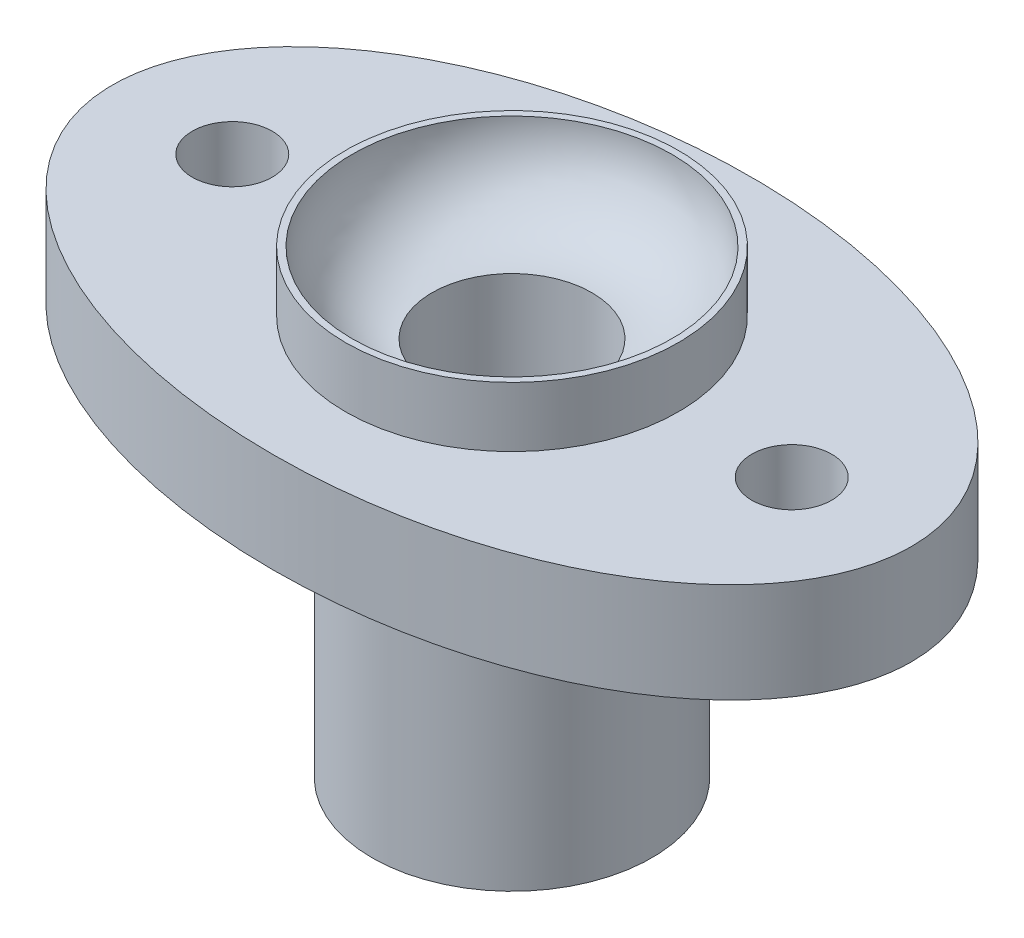
SolidWorks part; units mm, degrees
material "Plain Carbon Steel"
ref_plane "Front Plane" through (0, 0, 0) normal (0, 0, 1) x (1, 0, 0)
ref_plane "Top Plane" through (0, 0, 0) normal (0, 1, 0) x (1, 0, 0)
ref_plane "Right Plane" through (0, 0, 0) normal (1, 0, 0) x (0, 0, -1)
sketch "Shank Sketch Ø42" plane through (0, 0, 0) normal (0, 1, 0) x (1, 0, 0)
  circle A0 centre (0, 0) radius 21
  dimension "D1" = 42
extrude "Shank Ø42" add sketch "Shank Sketch Ø42" along normal blind 45
sketch "Flange Sketch 120x36" plane through (0, 45, 0) normal (0, 1, 0) x (1, 0, 0)
  ellipse E0 centre (0, 0) end of major axis (60, 0) minor radius 36
  dimension "D1" = 36
  dimension "D2" = 120
extrude "Oval Flange 120x36" add sketch "Flange Sketch 120x36" along normal blind 15
sketch "Spigot Sketch Ø50" plane through (0, 60, 0) normal (0, 1, 0) x (1, 0, 0)
  circle A0 centre (0, 0) radius 25
  dimension "D1" = 50
extrude "Spigot Ø50" add sketch "Spigot Sketch Ø50" along normal blind 9
sketch "Bore Profile Sketch" plane through (0, 0, 0) normal (0, 0, 1) x (1, 0, 0)
  line L0 (21, 0) -> (12, 2.4115)
  line L1 (12, 2.4115) -> (12, 57)
  line L2 (25, 69) -> (-25, 69) construction
  line L3 (-21, 0) -> (21, 0) construction
  line L4 (21, 0) -> (0, 0)
  line L5 (0, 0) -> (0, 69)
  line L6 (0, 69) -> (24, 69)
  arc A0 (12, 57) -> (24, 69) centre (12, 69) ccw
  dimension "D1" = 15
  dimension "D4" = 12
  dimension "D2" = 12
  dimension "D3" = 12
revolve "Bore and Seat Cut" cut sketch "Bore Profile Sketch" angle 360 about L5
sketch "Mounting Holes Sketch" plane through (0, 60, 0) normal (0, 1, 0) x (1, 0, 0)
  circle A0 centre (-42, 0) radius 6
  circle A1 centre (42, 0) radius 6
  dimension "D1" = 12
  dimension "D4" = 12
  dimension "D2" = 84
  dimension "D3" = 42
extrude "Mounting Holes 2xØ12" cut sketch "Mounting Holes Sketch" against normal blind 19
